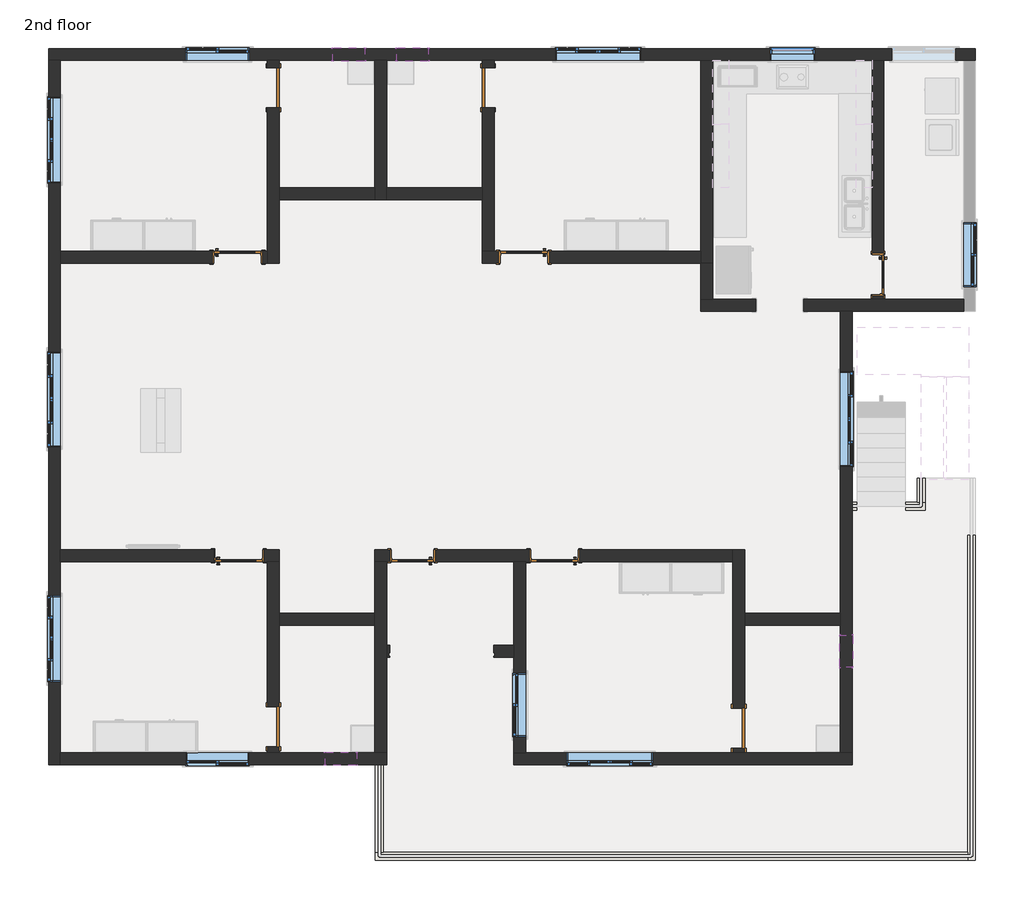
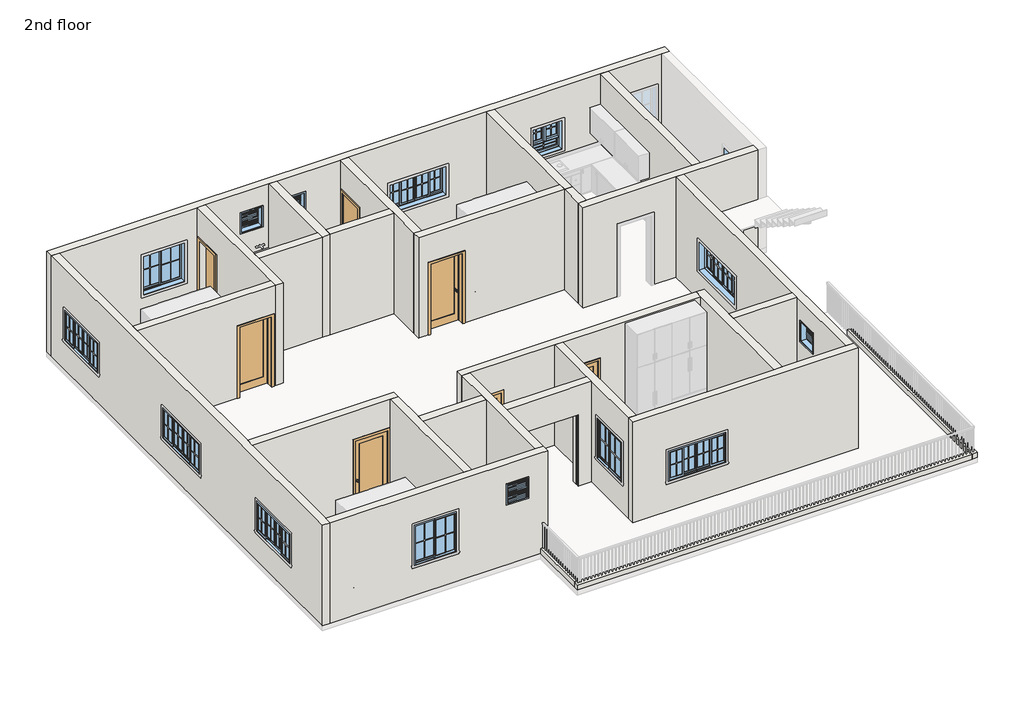
# One storey, part 1 of 4: 31 walls, 15 windows, 10 doors.
"""IFC4 building model written with IfcOpenShell, lengths in millimetres."""

from ifc_helpers import new_model, si_unit, frame, origin, place, context, project, spatial, polyline, outline, extrude, faceted_brep, transform, mapped, element, save
from components import door_ac3c0746, door_868ee8a9, door_3b97b8e7, door_c0815308, door_5e1232af, door_bb98abfd, window_ced37e8f, window_f2d8fef0, window_5af5dca6, window_95c4569f, window_58cce754

model = new_model("IFC4")

# Units and contexts
model_context = context("Model", 3, world=origin())
ifc_project = project(units=[si_unit("LENGTHUNIT", "METRE", prefix="MILLI")], contexts=[model_context])

# Site, building, storey
site = spatial("IfcSite", under=ifc_project)
building = spatial("IfcBuilding", under=site)
storey = spatial("IfcBuildingStorey", under=building, Name="2nd floor", Elevation=7010.4)

# Doors
placement = place(None, origin())
door_shape = door_ac3c0746(model_context)
element("IfcDoor", 1, ObjectType="Door-Interior-Single-1_Panel-Wood : 30\" x 84\"", at=placement, inside=storey, context=model_context, shape_type="MappedRepresentation", body=[
    mapped(door_shape, transform((7861.3010838, 2743.2660813, 7010.4), x_axis=(0.0, -1.0, 0.0), y_axis=(1.0, 0.0, 0.0), z_axis=(0.0, 0.0, 1.0))),
])
door_2_shape = door_868ee8a9(model_context)
element("IfcDoor", 2, ObjectType="Door-Interior-Single-1_Panel-Wood : 36\" x 84\"", at=placement, inside=storey, context=model_context, shape_type="MappedRepresentation", body=[
    mapped(door_2_shape, transform((1076.3260838, 3076.6410813, 7010.4), x_axis=(-1.0, 0.0, 0.0), y_axis=(0.0, -1.0, 0.0), z_axis=(0.0, 0.0, 1.0))),
])
element("IfcDoor", 3, ObjectType="Door-Interior-Single-1_Panel-Wood : 36\" x 84\"", at=placement, inside=storey, context=model_context, shape_type="MappedRepresentation", body=[
    mapped(door_2_shape, transform((-4384.6739162, -2644.7089187, 7010.4), x_axis=(1.0, 0.0, 0.0), y_axis=(0.0, 1.0, 0.0), z_axis=(0.0, 0.0, 1.0))),
])
door_3_shape = door_3b97b8e7(model_context)
element("IfcDoor", 4, ObjectType="Door-Interior-Single-1_Panel-Wood : 36\" x 84\"", at=placement, inside=storey, context=model_context, shape_type="MappedRepresentation", body=[
    mapped(door_3_shape, transform((1660.5260838, -2644.7089187, 7010.4), x_axis=(-1.0, 0.0, 0.0), y_axis=(0.0, -1.0, 0.0), z_axis=(0.0, 0.0, 1.0))),
])
element("IfcDoor", 5, ObjectType="Door-Interior-Single-1_Panel-Wood : 36\" x 84\"", at=placement, inside=storey, context=model_context, shape_type="MappedRepresentation", body=[
    mapped(door_3_shape, transform((-4410.0739162, 3076.6410813, 7010.4), x_axis=(1.0, 0.0, 0.0), y_axis=(0.0, 1.0, 0.0), z_axis=(0.0, 0.0, 1.0))),
])
door_4_shape = door_c0815308(model_context)
element("IfcDoor", 6, ObjectType="Door-Interior-Single-Full Glass-Wood : 32\" x 84\"", at=placement, inside=storey, context=model_context, shape_type="MappedRepresentation", body=[
    mapped(door_4_shape, transform((-1057.2739162, -2644.7089187, 7010.4), x_axis=(-1.0, 0.0, 0.0), y_axis=(0.0, -1.0, 0.0), z_axis=(0.0, 0.0, 1.0))),
])
door_5_shape = door_5e1232af(model_context)
element("IfcDoor", 7, ObjectType="Single-Flush : 30\" x 84\"", at=placement, inside=storey, context=model_context, shape_type="MappedRepresentation", body=[
    mapped(door_5_shape, transform((-3724.2739162, 6324.6660813, 7010.4), x_axis=(0.0, 1.0, 0.0), y_axis=(-1.0, 0.0, 0.0), z_axis=(0.0, 0.0, 1.0))),
])
door_6_shape = door_bb98abfd(model_context)
element("IfcDoor", 8, ObjectType="Single-Flush : 30\" x 84\"", at=placement, inside=storey, context=model_context, shape_type="MappedRepresentation", body=[
    mapped(door_6_shape, transform((390.5260838, 6324.6660813, 7010.4), x_axis=(0.0, 1.0, 0.0), y_axis=(-1.0, 0.0, 0.0), z_axis=(0.0, 0.0, 1.0))),
])
element("IfcDoor", 9, ObjectType="Single-Flush : 30\" x 84\"", at=placement, inside=storey, context=model_context, shape_type="MappedRepresentation", body=[
    mapped(door_6_shape, transform((-3724.2739162, -5918.1339187, 7010.4), x_axis=(0.0, -1.0, 0.0), y_axis=(1.0, 0.0, 0.0), z_axis=(0.0, 0.0, 1.0))),
])
element("IfcDoor", 10, ObjectType="Single-Flush : 30\" x 84\"", at=placement, inside=storey, context=model_context, shape_type="MappedRepresentation", body=[
    mapped(door_6_shape, transform((5191.1260838, -5943.5339187, 7010.4), x_axis=(0.0, -1.0, 0.0), y_axis=(1.0, 0.0, 0.0), z_axis=(0.0, 0.0, 1.0))),
])

# Walls
element("IfcWall", 11, ObjectType="Generic - 6\"", at=placement, inside=storey, context=model_context, shape_type="Brep", body=[
    faceted_brep([(9572.6260838, -8470.8339187, 7010.4), (9572.6260838, -8470.8339187, 7162.8), (9572.6260838, -8318.4339187, 7162.8), (9572.6260838, -2247.8339187, 7162.8), (9572.6260838, -2247.8339187, 7010.4), (9572.6260838, -8318.4339187, 7010.4), (9725.0260838, -8470.8339187, 7162.8), (9725.0260838, -8470.8339187, 7010.4), (9725.0260838, -2247.8339187, 7010.4), (9725.0260838, -2247.8339187, 7162.8)], [[[0, 1, 2, 3, 4, 5]], [[6, 7, 8, 9]], [[7, 0, 5, 4, 8]], [[1, 6, 9, 3, 2]], [[1, 0, 7, 6]], [[4, 3, 9, 8]]]),
])
element("IfcWall", 12, ObjectType="Generic - 6\"", at=placement, inside=storey, context=model_context, shape_type="Brep", body=[
    faceted_brep([(9572.6260838, -8318.4339187, 7010.4), (-1616.0739162, -8318.4339187, 7010.4), (-1768.4739162, -8318.4339187, 7010.4), (-1768.4739162, -8318.4339187, 7162.8), (-1616.0739162, -8318.4339187, 7162.8), (9572.6260838, -8318.4339187, 7162.8), (9572.6260838, -8470.8339187, 7010.4), (9572.6260838, -8470.8339187, 7162.8), (-1768.4739162, -8470.8339187, 7162.8), (-1768.4739162, -8470.8339187, 7010.4)], [[[0, 1, 2, 3, 4, 5]], [[6, 7, 8, 9]], [[2, 1, 0, 6, 9]], [[5, 4, 3, 8, 7]], [[0, 5, 7, 6]], [[3, 2, 9, 8]]]),
])
element("IfcWall", 13, ObjectType="Generic - 6\"", at=placement, inside=storey, context=model_context, shape_type="SweptSolid", body=[
    extrude(outline(polyline([(-1616.0739162, -6642.0339187), (-1616.0739162, -8318.4339187), (-1768.4739162, -8318.4339187), (-1768.4739162, -6642.0339187), (-1616.0739162, -6642.0339187)])), frame((0.0, 0.0, 7010.4), z_axis=(0.0, 0.0, 1.0), x_axis=(1.0, 0.0, 0.0)), (0.0, 0.0, 1.0), 152.4),
])
element("IfcWall", 14, ObjectType="Generic - 6\"", at=placement, inside=storey, context=model_context, shape_type="SweptSolid", body=[
    extrude(outline(polyline([(8607.4260838, -1612.8339187), (8607.4260838, -1156.9972984), (8759.8260838, -1156.9972984), (8759.8260838, -1612.8339187), (8607.4260838, -1612.8339187)])), frame((0.0, 0.0, 7010.4), z_axis=(0.0, 0.0, 1.0), x_axis=(1.0, 0.0, 0.0)), (0.0, 0.0, 1.0), 152.4),
])
element("IfcWall", 15, ObjectType="Generic - 6\"", at=placement, inside=storey, context=model_context, shape_type="Brep", body=[
    faceted_brep([(8759.8260838, -1612.8339187, 7010.4), (8607.4260838, -1612.8339187, 7010.4), (8391.5260838, -1612.8339187, 7010.4), (8391.5260838, -1612.8339187, 7162.8), (8607.4260838, -1612.8339187, 7162.8), (8759.8260838, -1612.8339187, 7162.8), (8759.8260838, -1765.2339187, 7010.4), (8759.8260838, -1765.2339187, 7162.8), (8391.5260838, -1765.2339187, 7162.8), (8391.5260838, -1765.2339187, 7010.4)], [[[0, 1, 2, 3, 4, 5]], [[6, 7, 8, 9]], [[2, 1, 0, 6, 9]], [[3, 2, 9, 8]], [[5, 4, 3, 8, 7]], [[0, 5, 7, 6]]]),
])
element("IfcWall", 16, ObjectType="Generic - 6\"", at=placement, inside=storey, context=model_context, shape_type="SweptSolid", body=[
    extrude(outline(polyline([(7362.8260838, -1612.8339187), (7451.7260838, -1612.8339187), (7451.7260838, -1765.2339187), (7362.8260838, -1765.2339187), (7362.8260838, -1612.8339187)])), frame((0.0, 0.0, 7010.4), z_axis=(0.0, 0.0, 1.0), x_axis=(1.0, 0.0, 0.0)), (0.0, 0.0, 1.0), 152.4),
])
element("IfcWall", 17, ObjectType="Generic - 9\"", at=placement, inside=storey, context=model_context, shape_type="Brep", body=[
    faceted_brep([(-8029.5739162, 6845.3660813, 7010.4), (-7800.9739162, 6845.3660813, 7010.4), (-3838.5739162, 6845.3660813, 7010.4), (-3609.9739162, 6845.3660813, 7010.4), (-1781.1739162, 6845.3660813, 7010.4), (-1552.5739162, 6845.3660813, 7010.4), (276.2260838, 6845.3660813, 7010.4), (504.8260838, 6845.3660813, 7010.4), (4467.2260838, 6845.3660813, 7010.4), (4695.8260838, 6845.3660813, 7010.4), (7743.8260838, 6845.3660813, 7010.4), (7972.4260838, 6845.3660813, 7010.4), (9496.4260838, 6845.3660813, 7010.4), (9725.0260838, 6845.3660813, 7010.4), (9725.0260838, 6845.3660813, 10058.4), (9496.4260838, 6845.3660813, 10058.4), (7972.4260838, 6845.3660813, 10058.4), (7743.8260838, 6845.3660813, 10058.4), (4695.8260838, 6845.3660813, 10058.4), (4467.2260838, 6845.3660813, 10058.4), (504.8260838, 6845.3660813, 10058.4), (276.2260838, 6845.3660813, 10058.4), (-1552.5739162, 6845.3660813, 10058.4), (-1781.1739162, 6845.3660813, 10058.4), (-3609.9739162, 6845.3660813, 10058.4), (-3838.5739162, 6845.3660813, 10058.4), (-7800.9739162, 6845.3660813, 10058.4), (-8029.5739162, 6845.3660813, 10058.4), (3324.2260838, 6845.3660813, 8839.2), (3324.2260838, 6845.3660813, 7924.8), (1673.2260838, 6845.3660813, 7924.8), (1673.2260838, 6845.3660813, 8839.2), (9344.0260838, 6845.3660813, 9144.0), (9344.0260838, 6845.3660813, 7924.8), (8124.8260838, 6845.3660813, 7924.8), (8124.8260838, 6845.3660813, 9144.0), (-2581.2739162, 6845.3660813, 9448.8), (-1971.6739162, 6845.3660813, 9448.8), (-1971.6739162, 6845.3660813, 8839.2), (-2581.2739162, 6845.3660813, 8839.2), (-1362.0739162, 6845.3660813, 9448.8), (-752.4739162, 6845.3660813, 9448.8), (-752.4739162, 6845.3660813, 8839.2), (-1362.0739162, 6845.3660813, 8839.2), (-4181.4739162, 6845.3660813, 9144.0), (-4181.4739162, 6845.3660813, 7924.8), (-5400.6739162, 6845.3660813, 7924.8), (-5400.6739162, 6845.3660813, 9144.0), (6651.6260838, 6845.3660813, 9067.8), (6651.6260838, 6845.3660813, 8153.4), (5788.0260838, 6845.3660813, 8153.4), (5788.0260838, 6845.3660813, 9067.8), (-8029.5739162, 7073.9660813, 7010.4), (-8029.5739162, 7073.9660813, 10058.4), (9725.0260838, 7073.9660813, 10058.4), (9725.0260838, 7073.9660813, 7010.4), (3324.2260838, 7073.9660813, 8839.2), (1673.2260838, 7073.9660813, 8839.2), (1673.2260838, 7073.9660813, 7924.8), (3324.2260838, 7073.9660813, 7924.8), (9344.0260838, 7073.9660813, 9144.0), (8124.8260838, 7073.9660813, 9144.0), (8124.8260838, 7073.9660813, 7924.8), (9344.0260838, 7073.9660813, 7924.8), (-2581.2739162, 7073.9660813, 9448.8), (-2581.2739162, 7073.9660813, 8839.2), (-1971.6739162, 7073.9660813, 8839.2), (-1971.6739162, 7073.9660813, 9448.8), (-1362.0739162, 7073.9660813, 9448.8), (-1362.0739162, 7073.9660813, 8839.2), (-752.4739162, 7073.9660813, 8839.2), (-752.4739162, 7073.9660813, 9448.8), (-4181.4739162, 7073.9660813, 9144.0), (-5400.6739162, 7073.9660813, 9144.0), (-5400.6739162, 7073.9660813, 7924.8), (-4181.4739162, 7073.9660813, 7924.8), (6651.6260838, 7073.9660813, 9067.8), (5788.0260838, 7073.9660813, 9067.8), (5788.0260838, 7073.9660813, 8153.4), (6651.6260838, 7073.9660813, 8153.4)], [[[0, 1, 2, 3, 4, 5, 6, 7, 8, 9, 10, 11, 12, 13, 14, 15, 16, 17, 18, 19, 20, 21, 22, 23, 24, 25, 26, 27], [28, 29, 30, 31], [32, 33, 34, 35], [36, 37, 38, 39], [40, 41, 42, 43], [44, 45, 46, 47], [48, 49, 50, 51]], [[52, 53, 54, 55], [56, 57, 58, 59], [60, 61, 62, 63], [64, 65, 66, 67], [68, 69, 70, 71], [72, 73, 74, 75], [76, 77, 78, 79]], [[13, 12, 11, 10, 9, 8, 7, 6, 5, 4, 3, 2, 1, 0, 52, 55]], [[0, 27, 53, 52]], [[14, 13, 55, 54]], [[29, 28, 56, 59]], [[30, 29, 59, 58]], [[31, 30, 58, 57]], [[28, 31, 57, 56]], [[33, 32, 60, 63]], [[34, 33, 63, 62]], [[35, 34, 62, 61]], [[32, 35, 61, 60]], [[65, 64, 36, 39]], [[66, 65, 39, 38]], [[67, 66, 38, 37]], [[64, 67, 37, 36]], [[69, 68, 40, 43]], [[70, 69, 43, 42]], [[71, 70, 42, 41]], [[68, 71, 41, 40]], [[45, 44, 72, 75]], [[46, 45, 75, 74]], [[47, 46, 74, 73]], [[44, 47, 73, 72]], [[49, 48, 76, 79]], [[50, 49, 79, 78]], [[51, 50, 78, 77]], [[48, 51, 77, 76]], [[27, 26, 25, 24, 23, 22, 21, 20, 19, 18, 17, 16, 15, 14, 54, 53]]]),
])
element("IfcWall", 18, ObjectType="Generic - 9\"", at=placement, inside=storey, context=model_context, shape_type="Brep", body=[
    faceted_brep([(-8029.5739162, 6845.3660813, 7010.4), (-8029.5739162, -6642.0339187, 7010.4), (-8029.5739162, -6642.0339187, 10058.4), (-8029.5739162, 6845.3660813, 10058.4), (-8029.5739162, 1270.0660813, 8839.2), (-8029.5739162, -558.7339187, 8839.2), (-8029.5739162, -558.7339187, 7924.8), (-8029.5739162, 1270.0660813, 7924.8), (-8029.5739162, 6146.8660813, 8839.2), (-8029.5739162, 4495.8660813, 8839.2), (-8029.5739162, 4495.8660813, 7924.8), (-8029.5739162, 6146.8660813, 7924.8), (-8029.5739162, -3403.5339187, 8839.2), (-8029.5739162, -5054.5339187, 8839.2), (-8029.5739162, -5054.5339187, 7924.8), (-8029.5739162, -3403.5339187, 7924.8), (-7800.9739162, 6845.3660813, 7010.4), (-7800.9739162, 6845.3660813, 10058.4), (-7800.9739162, 3187.7660813, 10058.4), (-7800.9739162, 2959.1660813, 10058.4), (-7800.9739162, -2527.2339187, 10058.4), (-7800.9739162, -2755.8339187, 10058.4), (-7800.9739162, -6413.4339187, 10058.4), (-7800.9739162, -6642.0339187, 10058.4), (-7800.9739162, -6642.0339187, 7010.4), (-7800.9739162, -6413.4339187, 7010.4), (-7800.9739162, -2755.8339187, 7010.4), (-7800.9739162, -2527.2339187, 7010.4), (-7800.9739162, 2959.1660813, 7010.4), (-7800.9739162, 3187.7660813, 7010.4), (-7800.9739162, 1270.0660813, 8839.2), (-7800.9739162, 1270.0660813, 7924.8), (-7800.9739162, -558.7339187, 7924.8), (-7800.9739162, -558.7339187, 8839.2), (-7800.9739162, 6146.8660813, 8839.2), (-7800.9739162, 6146.8660813, 7924.8), (-7800.9739162, 4495.8660813, 7924.8), (-7800.9739162, 4495.8660813, 8839.2), (-7800.9739162, -3403.5339187, 8839.2), (-7800.9739162, -3403.5339187, 7924.8), (-7800.9739162, -5054.5339187, 7924.8), (-7800.9739162, -5054.5339187, 8839.2)], [[[0, 1, 2, 3], [4, 5, 6, 7], [8, 9, 10, 11], [12, 13, 14, 15]], [[16, 17, 18, 19, 20, 21, 22, 23, 24, 25, 26, 27, 28, 29], [30, 31, 32, 33], [34, 35, 36, 37], [38, 39, 40, 41]], [[1, 0, 16, 29, 28, 27, 26, 25, 24]], [[0, 3, 17, 16]], [[2, 1, 24, 23]], [[31, 30, 4, 7]], [[32, 31, 7, 6]], [[33, 32, 6, 5]], [[30, 33, 5, 4]], [[35, 34, 8, 11]], [[36, 35, 11, 10]], [[37, 36, 10, 9]], [[34, 37, 9, 8]], [[39, 38, 12, 15]], [[40, 39, 15, 14]], [[41, 40, 14, 13]], [[38, 41, 13, 12]], [[3, 2, 23, 22, 21, 20, 19, 18, 17]]]),
])
element("IfcWall", 19, ObjectType="Generic - 9\"", at=placement, inside=storey, context=model_context, shape_type="Brep", body=[
    faceted_brep([(-3838.5739162, 6845.3660813, 10058.4), (-3838.5739162, 6845.3660813, 7010.4), (-3838.5739162, 6705.6660813, 7010.4), (-3838.5739162, 6705.6660813, 9144.0), (-3838.5739162, 5943.6660813, 9144.0), (-3838.5739162, 5943.6660813, 7010.4), (-3838.5739162, 3187.7660813, 7010.4), (-3838.5739162, 2959.1660813, 7010.4), (-3838.5739162, 2959.1660813, 10058.4), (-3838.5739162, 3187.7660813, 10058.4), (-3609.9739162, 6845.3660813, 7010.4), (-3609.9739162, 6845.3660813, 10058.4), (-3609.9739162, 4406.9660813, 10058.4), (-3609.9739162, 4178.3660813, 10058.4), (-3609.9739162, 2959.1660813, 10058.4), (-3609.9739162, 2959.1660813, 7010.4), (-3609.9739162, 4178.3660813, 7010.4), (-3609.9739162, 4406.9660813, 7010.4), (-3609.9739162, 5943.6660813, 7010.4), (-3609.9739162, 5943.6660813, 9144.0), (-3609.9739162, 6705.6660813, 9144.0), (-3609.9739162, 6705.6660813, 7010.4)], [[[0, 1, 2, 3, 4, 5, 6, 7, 8, 9]], [[10, 11, 12, 13, 14, 15, 16, 17, 18, 19, 20, 21]], [[1, 10, 21, 2]], [[15, 7, 6, 5, 18, 17, 16]], [[1, 0, 11, 10]], [[8, 7, 15, 14]], [[20, 3, 2, 21]], [[4, 19, 18, 5]], [[19, 4, 3, 20]], [[0, 9, 8, 14, 13, 12, 11]]]),
])
element("IfcWall", 20, ObjectType="Generic - 9\"", at=placement, inside=storey, context=model_context, shape_type="Brep", body=[
    faceted_brep([(-1781.1739162, 6845.3660813, 7010.4), (-1781.1739162, 4406.9660813, 7010.4), (-1781.1739162, 4178.3660813, 7010.4), (-1781.1739162, 4178.3660813, 10058.4), (-1781.1739162, 4406.9660813, 10058.4), (-1781.1739162, 6845.3660813, 10058.4), (-1552.5739162, 6845.3660813, 7010.4), (-1552.5739162, 6845.3660813, 10058.4), (-1552.5739162, 4406.9660813, 10058.4), (-1552.5739162, 4178.3660813, 10058.4), (-1552.5739162, 4178.3660813, 7010.4), (-1552.5739162, 4406.9660813, 7010.4)], [[[0, 1, 2, 3, 4, 5]], [[6, 7, 8, 9, 10, 11]], [[2, 1, 0, 6, 11, 10]], [[0, 5, 7, 6]], [[3, 2, 10, 9]], [[5, 4, 3, 9, 8, 7]]]),
])
element("IfcWall", 21, ObjectType="Generic - 9\"", at=placement, inside=storey, context=model_context, shape_type="Brep", body=[
    faceted_brep([(276.2260838, 6845.3660813, 10058.4), (276.2260838, 6845.3660813, 7010.4), (276.2260838, 6705.6660813, 7010.4), (276.2260838, 6705.6660813, 9144.0), (276.2260838, 5943.6660813, 9144.0), (276.2260838, 5943.6660813, 7010.4), (276.2260838, 4406.9660813, 7010.4), (276.2260838, 4178.3660813, 7010.4), (276.2260838, 3187.7660813, 7010.4), (276.2260838, 3187.7660813, 10058.4), (276.2260838, 4178.3660813, 10058.4), (276.2260838, 4406.9660813, 10058.4), (504.8260838, 6845.3660813, 7010.4), (504.8260838, 6845.3660813, 10058.4), (504.8260838, 3187.7660813, 10058.4), (504.8260838, 3187.7660813, 7010.4), (504.8260838, 5943.6660813, 7010.4), (504.8260838, 5943.6660813, 9144.0), (504.8260838, 6705.6660813, 9144.0), (504.8260838, 6705.6660813, 7010.4)], [[[0, 1, 2, 3, 4, 5, 6, 7, 8, 9, 10, 11]], [[12, 13, 14, 15, 16, 17, 18, 19]], [[1, 12, 19, 2]], [[15, 8, 7, 6, 5, 16]], [[1, 0, 13, 12]], [[9, 8, 15, 14]], [[18, 3, 2, 19]], [[4, 17, 16, 5]], [[17, 4, 3, 18]], [[0, 11, 10, 9, 14, 13]]]),
])
element("IfcWall", 22, ObjectType="Generic - 9\"", at=placement, inside=storey, context=model_context, shape_type="Brep", body=[
    faceted_brep([(4467.2260838, 6845.3660813, 7010.4), (4467.2260838, 3187.7660813, 7010.4), (4467.2260838, 2959.1660813, 7010.4), (4467.2260838, 2959.1660813, 10058.4), (4467.2260838, 3187.7660813, 10058.4), (4467.2260838, 6845.3660813, 10058.4), (4695.8260838, 6845.3660813, 7010.4), (4695.8260838, 6845.3660813, 10058.4), (4695.8260838, 2959.1660813, 10058.4), (4695.8260838, 2959.1660813, 7010.4)], [[[0, 1, 2, 3, 4, 5]], [[6, 7, 8, 9]], [[2, 1, 0, 6, 9]], [[3, 2, 9, 8]], [[0, 5, 7, 6]], [[5, 4, 3, 8, 7]]]),
])
element("IfcWall", 23, ObjectType="Generic - 9\"", at=placement, inside=storey, context=model_context, shape_type="SweptSolid", body=[
    extrude(outline(polyline([(7010.4, -3838.5739162), (10058.4, -3838.5739162), (10058.4, -7800.9739162), (7010.4, -7800.9739162), (7010.4, -4892.6739162), (9169.4, -4892.6739162), (9169.4, -3927.4739162), (7010.4, -3927.4739162), (7010.4, -3838.5739162)])), frame((0.0, 2959.1660813, 0.0), z_axis=(0.0, 1.0, 0.0), x_axis=(0.0, 0.0, 1.0)), (0.0, 0.0, 1.0), 228.6),
])
element("IfcWall", 24, ObjectType="Generic - 9\"", at=placement, inside=storey, context=model_context, shape_type="SweptSolid", body=[
    extrude(outline(polyline([(-3609.9739162, 4406.9660813), (-1781.1739162, 4406.9660813), (-1781.1739162, 4178.3660813), (-3609.9739162, 4178.3660813), (-3609.9739162, 4406.9660813)])), frame((0.0, 0.0, 7010.4), z_axis=(0.0, 0.0, 1.0), x_axis=(1.0, 0.0, 0.0)), (0.0, 0.0, 1.0), 3048.0),
])
element("IfcWall", 25, ObjectType="Generic - 9\"", at=placement, inside=storey, context=model_context, shape_type="SweptSolid", body=[
    extrude(outline(polyline([(276.2260838, 4178.3660813), (-1552.5739162, 4178.3660813), (-1552.5739162, 4406.9660813), (276.2260838, 4406.9660813), (276.2260838, 4178.3660813)])), frame((0.0, 0.0, 7010.4), z_axis=(0.0, 0.0, 1.0), x_axis=(1.0, 0.0, 0.0)), (0.0, 0.0, 1.0), 3048.0),
])
element("IfcWall", 26, ObjectType="Generic - 9\"", at=placement, inside=storey, context=model_context, shape_type="Brep", body=[
    faceted_brep([(4467.2260838, 2959.1660813, 7010.4), (4467.2260838, 2959.1660813, 10058.4), (276.2260838, 2959.1660813, 10058.4), (276.2260838, 2959.1660813, 7010.4), (593.7260838, 2959.1660813, 7010.4), (593.7260838, 2959.1660813, 9169.4), (1558.9260838, 2959.1660813, 9169.4), (1558.9260838, 2959.1660813, 7010.4), (4467.2260838, 3187.7660813, 10058.4), (4467.2260838, 3187.7660813, 7010.4), (1558.9260838, 3187.7660813, 7010.4), (1558.9260838, 3187.7660813, 9169.4), (593.7260838, 3187.7660813, 9169.4), (593.7260838, 3187.7660813, 7010.4), (504.8260838, 3187.7660813, 7010.4), (276.2260838, 3187.7660813, 7010.4), (276.2260838, 3187.7660813, 10058.4), (504.8260838, 3187.7660813, 10058.4)], [[[0, 1, 2, 3, 4, 5, 6, 7]], [[8, 9, 10, 11, 12, 13, 14, 15, 16, 17]], [[9, 0, 7, 10]], [[3, 15, 14, 13, 4]], [[1, 0, 9, 8]], [[3, 2, 16, 15]], [[12, 5, 4, 13]], [[5, 12, 11, 6]], [[6, 11, 10, 7]], [[2, 1, 8, 17, 16]]]),
])
element("IfcWall", 27, ObjectType="Generic - 9\"", at=placement, inside=storey, context=model_context, shape_type="Brep", body=[
    faceted_brep([(-7800.9739162, -2755.8339187, 10058.4), (-7800.9739162, -2755.8339187, 7010.4), (-4867.2739162, -2755.8339187, 7010.4), (-4867.2739162, -2755.8339187, 9169.4), (-3902.0739162, -2755.8339187, 9169.4), (-3902.0739162, -2755.8339187, 7010.4), (-3838.5739162, -2755.8339187, 7010.4), (-3609.9739162, -2755.8339187, 7010.4), (-3609.9739162, -2755.8339187, 10058.4), (-3838.5739162, -2755.8339187, 10058.4), (-7800.9739162, -2527.2339187, 7010.4), (-7800.9739162, -2527.2339187, 10058.4), (-3609.9739162, -2527.2339187, 10058.4), (-3609.9739162, -2527.2339187, 7010.4), (-3902.0739162, -2527.2339187, 7010.4), (-3902.0739162, -2527.2339187, 9169.4), (-4867.2739162, -2527.2339187, 9169.4), (-4867.2739162, -2527.2339187, 7010.4)], [[[0, 1, 2, 3, 4, 5, 6, 7, 8, 9]], [[10, 11, 12, 13, 14, 15, 16, 17]], [[1, 10, 17, 2]], [[13, 7, 6, 5, 14]], [[1, 0, 11, 10]], [[8, 7, 13, 12]], [[4, 15, 14, 5]], [[15, 4, 3, 16]], [[16, 3, 2, 17]], [[0, 9, 8, 12, 11]]]),
])
element("IfcWall", 28, ObjectType="Generic - 9\"", at=placement, inside=storey, context=model_context, shape_type="Brep", body=[
    faceted_brep([(-7800.9739162, -6642.0339187, 7010.4), (-1768.4739162, -6642.0339187, 7010.4), (-1616.0739162, -6642.0339187, 7010.4), (-1552.5739162, -6642.0339187, 7010.4), (-1552.5739162, -6642.0339187, 10058.4), (-1781.1739162, -6642.0339187, 10058.4), (-7800.9739162, -6642.0339187, 10058.4), (-5400.6739162, -6642.0339187, 7924.8), (-5400.6739162, -6642.0339187, 9144.0), (-4181.4739162, -6642.0339187, 9144.0), (-4181.4739162, -6642.0339187, 7924.8), (-2124.0739162, -6642.0339187, 9448.8), (-2124.0739162, -6642.0339187, 8839.2), (-2733.6739162, -6642.0339187, 8839.2), (-2733.6739162, -6642.0339187, 9448.8), (-1552.5739162, -6413.4339187, 7010.4), (-1781.1739162, -6413.4339187, 7010.4), (-3609.9739162, -6413.4339187, 7010.4), (-3838.5739162, -6413.4339187, 7010.4), (-7800.9739162, -6413.4339187, 7010.4), (-7800.9739162, -6413.4339187, 10058.4), (-3838.5739162, -6413.4339187, 10058.4), (-3609.9739162, -6413.4339187, 10058.4), (-1781.1739162, -6413.4339187, 10058.4), (-1552.5739162, -6413.4339187, 10058.4), (-5400.6739162, -6413.4339187, 9144.0), (-5400.6739162, -6413.4339187, 7924.8), (-4181.4739162, -6413.4339187, 7924.8), (-4181.4739162, -6413.4339187, 9144.0), (-2124.0739162, -6413.4339187, 8839.2), (-2124.0739162, -6413.4339187, 9448.8), (-2733.6739162, -6413.4339187, 9448.8), (-2733.6739162, -6413.4339187, 8839.2)], [[[0, 1, 2, 3, 4, 5, 6], [7, 8, 9, 10], [11, 12, 13, 14]], [[15, 16, 17, 18, 19, 20, 21, 22, 23, 24], [25, 26, 27, 28], [29, 30, 31, 32]], [[3, 2, 1, 0, 19, 18, 17, 16, 15]], [[0, 6, 20, 19]], [[25, 8, 7, 26]], [[26, 7, 10, 27]], [[27, 10, 9, 28]], [[8, 25, 28, 9]], [[12, 11, 30, 29]], [[13, 12, 29, 32]], [[14, 13, 32, 31]], [[11, 14, 31, 30]], [[3, 15, 24, 4]], [[24, 23, 22, 21, 20, 6, 5, 4]]]),
])
element("IfcWall", 29, ObjectType="Generic - 9\"", at=placement, inside=storey, context=model_context, shape_type="Brep", body=[
    faceted_brep([(-3609.9739162, -6413.4339187, 10058.4), (-3609.9739162, -6413.4339187, 7010.4), (-3609.9739162, -6299.1339187, 7010.4), (-3609.9739162, -6299.1339187, 9144.0), (-3609.9739162, -5537.1339187, 9144.0), (-3609.9739162, -5537.1339187, 7010.4), (-3609.9739162, -3975.0339187, 7010.4), (-3609.9739162, -3746.4339187, 7010.4), (-3609.9739162, -2755.8339187, 7010.4), (-3609.9739162, -2755.8339187, 10058.4), (-3609.9739162, -3746.4339187, 10058.4), (-3609.9739162, -3975.0339187, 10058.4), (-3838.5739162, -6413.4339187, 7010.4), (-3838.5739162, -6413.4339187, 10058.4), (-3838.5739162, -2755.8339187, 10058.4), (-3838.5739162, -2755.8339187, 7010.4), (-3838.5739162, -5537.1339187, 7010.4), (-3838.5739162, -5537.1339187, 9144.0), (-3838.5739162, -6299.1339187, 9144.0), (-3838.5739162, -6299.1339187, 7010.4)], [[[0, 1, 2, 3, 4, 5, 6, 7, 8, 9, 10, 11]], [[12, 13, 14, 15, 16, 17, 18, 19]], [[1, 12, 19, 2]], [[15, 8, 7, 6, 5, 16]], [[1, 0, 13, 12]], [[9, 8, 15, 14]], [[18, 3, 2, 19]], [[4, 17, 16, 5]], [[17, 4, 3, 18]], [[0, 11, 10, 9, 14, 13]]]),
])
element("IfcWall", 30, ObjectType="Generic - 9\"", at=placement, inside=storey, context=model_context, shape_type="Brep", body=[
    faceted_brep([(-1781.1739162, -2755.8339187, 7010.4), (-1781.1739162, -3746.4339187, 7010.4), (-1781.1739162, -3975.0339187, 7010.4), (-1781.1739162, -6413.4339187, 7010.4), (-1781.1739162, -6413.4339187, 10058.4), (-1781.1739162, -3975.0339187, 10058.4), (-1781.1739162, -3746.4339187, 10058.4), (-1781.1739162, -2755.8339187, 10058.4), (-1552.5739162, -2755.8339187, 7010.4), (-1552.5739162, -2755.8339187, 10058.4), (-1552.5739162, -4356.0339187, 10058.4), (-1552.5739162, -4584.6339187, 10058.4), (-1552.5739162, -6413.4339187, 10058.4), (-1552.5739162, -6413.4339187, 7010.4), (-1552.5739162, -4584.6339187, 7010.4), (-1552.5739162, -4356.0339187, 7010.4)], [[[0, 1, 2, 3, 4, 5, 6, 7]], [[8, 9, 10, 11, 12, 13, 14, 15]], [[3, 2, 1, 0, 8, 15, 14, 13]], [[0, 7, 9, 8]], [[7, 6, 5, 4, 12, 11, 10, 9]], [[3, 13, 12, 4]]]),
])
element("IfcWall", 31, ObjectType="Generic - 9\"", at=placement, inside=storey, context=model_context, shape_type="SweptSolid", body=[
    extrude(outline(polyline([(-3609.9739162, -3746.4339187), (-1781.1739162, -3746.4339187), (-1781.1739162, -3975.0339187), (-3609.9739162, -3975.0339187), (-3609.9739162, -3746.4339187)])), frame((0.0, 0.0, 7010.4), z_axis=(0.0, 0.0, 1.0), x_axis=(1.0, 0.0, 0.0)), (0.0, 0.0, 1.0), 3048.0),
])
element("IfcWall", 32, ObjectType="Generic - 9\"", at=placement, inside=storey, context=model_context, shape_type="Brep", body=[
    faceted_brep([(1114.4260838, -6413.4339187, 7010.4), (1114.4260838, -2755.8339187, 7010.4), (1114.4260838, -2755.8339187, 10058.4), (1114.4260838, -6413.4339187, 10058.4), (1114.4260838, -4889.4339187, 9144.0), (1114.4260838, -4889.4339187, 7924.8), (1114.4260838, -6108.6339187, 7924.8), (1114.4260838, -6108.6339187, 9144.0), (885.8260838, -2755.8339187, 7010.4), (885.8260838, -4356.0339187, 7010.4), (885.8260838, -4584.6339187, 7010.4), (885.8260838, -6413.4339187, 7010.4), (885.8260838, -6413.4339187, 10058.4), (885.8260838, -4584.6339187, 10058.4), (885.8260838, -4356.0339187, 10058.4), (885.8260838, -2755.8339187, 10058.4), (885.8260838, -4889.4339187, 7924.8), (885.8260838, -4889.4339187, 9144.0), (885.8260838, -6108.6339187, 9144.0), (885.8260838, -6108.6339187, 7924.8)], [[[0, 1, 2, 3], [4, 5, 6, 7]], [[8, 9, 10, 11, 12, 13, 14, 15], [16, 17, 18, 19]], [[1, 0, 11, 10, 9, 8]], [[2, 1, 8, 15]], [[0, 3, 12, 11]], [[4, 17, 16, 5]], [[5, 16, 19, 6]], [[6, 19, 18, 7]], [[17, 4, 7, 18]], [[3, 2, 15, 14, 13, 12]]]),
])
element("IfcWall", 33, ObjectType="Generic - 9\"", at=placement, inside=storey, context=model_context, shape_type="Brep", body=[
    faceted_brep([(-1781.1739162, -2527.2339187, 7010.4), (-1781.1739162, -2527.2339187, 10058.4), (5076.8260838, -2527.2339187, 10058.4), (5076.8260838, -2527.2339187, 7010.4), (2143.1260838, -2527.2339187, 7010.4), (2143.1260838, -2527.2339187, 9169.4), (1177.9260838, -2527.2339187, 9169.4), (1177.9260838, -2527.2339187, 7010.4), (-625.4739162, -2527.2339187, 7010.4), (-625.4739162, -2527.2339187, 9169.4), (-1489.0739162, -2527.2339187, 9169.4), (-1489.0739162, -2527.2339187, 7010.4), (-1781.1739162, -2755.8339187, 10058.4), (-1781.1739162, -2755.8339187, 7010.4), (-1552.5739162, -2755.8339187, 7010.4), (-1489.0739162, -2755.8339187, 7010.4), (-1489.0739162, -2755.8339187, 9169.4), (-625.4739162, -2755.8339187, 9169.4), (-625.4739162, -2755.8339187, 7010.4), (885.8260838, -2755.8339187, 7010.4), (1114.4260838, -2755.8339187, 7010.4), (1177.9260838, -2755.8339187, 7010.4), (1177.9260838, -2755.8339187, 9169.4), (2143.1260838, -2755.8339187, 9169.4), (2143.1260838, -2755.8339187, 7010.4), (5076.8260838, -2755.8339187, 7010.4), (5076.8260838, -2755.8339187, 10058.4), (1114.4260838, -2755.8339187, 10058.4), (885.8260838, -2755.8339187, 10058.4), (-1552.5739162, -2755.8339187, 10058.4)], [[[0, 1, 2, 3, 4, 5, 6, 7, 8, 9, 10, 11]], [[12, 13, 14, 15, 16, 17, 18, 19, 20, 21, 22, 23, 24, 25, 26, 27, 28, 29]], [[13, 0, 11, 15, 14]], [[3, 25, 24, 4]], [[7, 21, 20, 19, 18, 8]], [[1, 0, 13, 12]], [[3, 2, 26, 25]], [[6, 22, 21, 7]], [[22, 6, 5, 23]], [[23, 5, 4, 24]], [[10, 16, 15, 11]], [[16, 10, 9, 17]], [[17, 9, 8, 18]], [[2, 1, 12, 29, 28, 27, 26]]]),
])
element("IfcWall", 34, ObjectType="Generic - 9\"", at=placement, inside=storey, context=model_context, shape_type="Brep", body=[
    faceted_brep([(5305.4260838, -6413.4339187, 10058.4), (5305.4260838, -6413.4339187, 7010.4), (5305.4260838, -6324.5339187, 7010.4), (5305.4260838, -6324.5339187, 9144.0), (5305.4260838, -5562.5339187, 9144.0), (5305.4260838, -5562.5339187, 7010.4), (5305.4260838, -3975.0339187, 7010.4), (5305.4260838, -3746.4339187, 7010.4), (5305.4260838, -2527.2339187, 7010.4), (5305.4260838, -2527.2339187, 10058.4), (5305.4260838, -3746.4339187, 10058.4), (5305.4260838, -3975.0339187, 10058.4), (5076.8260838, -6413.4339187, 7010.4), (5076.8260838, -6413.4339187, 10058.4), (5076.8260838, -2755.8339187, 10058.4), (5076.8260838, -2527.2339187, 10058.4), (5076.8260838, -2527.2339187, 7010.4), (5076.8260838, -2755.8339187, 7010.4), (5076.8260838, -5562.5339187, 7010.4), (5076.8260838, -5562.5339187, 9144.0), (5076.8260838, -6324.5339187, 9144.0), (5076.8260838, -6324.5339187, 7010.4)], [[[0, 1, 2, 3, 4, 5, 6, 7, 8, 9, 10, 11]], [[12, 13, 14, 15, 16, 17, 18, 19, 20, 21]], [[1, 12, 21, 2]], [[16, 8, 7, 6, 5, 18, 17]], [[1, 0, 13, 12]], [[9, 8, 16, 15]], [[20, 3, 2, 21]], [[4, 19, 18, 5]], [[19, 4, 3, 20]], [[0, 11, 10, 9, 15, 14, 13]]]),
])
element("IfcWall", 35, ObjectType="Generic - 9\"", at=placement, inside=storey, context=model_context, shape_type="Brep", body=[
    faceted_brep([(7362.8260838, -6413.4339187, 7010.4), (7362.8260838, -1765.2339187, 7010.4), (7362.8260838, -1612.8339187, 7010.4), (7362.8260838, 2044.7660813, 7010.4), (7362.8260838, 2044.7660813, 10058.4), (7362.8260838, -1689.0339187, 10058.4), (7362.8260838, -6413.4339187, 10058.4), (7362.8260838, -939.7339187, 7924.8), (7362.8260838, -939.7339187, 8839.2), (7362.8260838, 889.0660813, 8839.2), (7362.8260838, 889.0660813, 7924.8), (7362.8260838, -4165.5339187, 9448.8), (7362.8260838, -4165.5339187, 8839.2), (7362.8260838, -4775.1339187, 8839.2), (7362.8260838, -4775.1339187, 9448.8), (7134.2260838, 2044.7660813, 7010.4), (7134.2260838, -3746.4339187, 7010.4), (7134.2260838, -3975.0339187, 7010.4), (7134.2260838, -6413.4339187, 7010.4), (7134.2260838, -6413.4339187, 10058.4), (7134.2260838, -3975.0339187, 10058.4), (7134.2260838, -3746.4339187, 10058.4), (7134.2260838, 2044.7660813, 10058.4), (7134.2260838, -939.7339187, 8839.2), (7134.2260838, -939.7339187, 7924.8), (7134.2260838, 889.0660813, 7924.8), (7134.2260838, 889.0660813, 8839.2), (7134.2260838, -4165.5339187, 8839.2), (7134.2260838, -4165.5339187, 9448.8), (7134.2260838, -4775.1339187, 9448.8), (7134.2260838, -4775.1339187, 8839.2)], [[[0, 1, 2, 3, 4, 5, 6], [7, 8, 9, 10], [11, 12, 13, 14]], [[15, 16, 17, 18, 19, 20, 21, 22], [23, 24, 25, 26], [27, 28, 29, 30]], [[3, 2, 1, 0, 18, 17, 16, 15]], [[4, 3, 15, 22]], [[0, 6, 19, 18]], [[23, 8, 7, 24]], [[24, 7, 10, 25]], [[25, 10, 9, 26]], [[8, 23, 26, 9]], [[12, 11, 28, 27]], [[13, 12, 27, 30]], [[14, 13, 30, 29]], [[11, 14, 29, 28]], [[22, 21, 20, 19, 6, 5, 4]]]),
])
element("IfcWall", 36, ObjectType="Generic - 9\"", at=placement, inside=storey, context=model_context, shape_type="SweptSolid", body=[
    extrude(outline(polyline([(5305.4260838, -3746.4339187), (7134.2260838, -3746.4339187), (7134.2260838, -3975.0339187), (5305.4260838, -3975.0339187), (5305.4260838, -3746.4339187)])), frame((0.0, 0.0, 7010.4), z_axis=(0.0, 0.0, 1.0), x_axis=(1.0, 0.0, 0.0)), (0.0, 0.0, 1.0), 3048.0),
])
element("IfcWall", 37, ObjectType="Generic - 9\"", at=placement, inside=storey, context=model_context, shape_type="SweptSolid", body=[
    extrude(outline(polyline([(6845.3660813, 10058.4), (6845.3660813, 7010.4), (3149.6660813, 7010.4), (3149.6660813, 9169.4), (2336.8660813, 9169.4), (2336.8660813, 7010.4), (2273.3660813, 7010.4), (2273.3660813, 10058.4), (6845.3660813, 10058.4)])), frame((7743.8260838, 0.0, 0.0), z_axis=(1.0, 0.0, 0.0), x_axis=(0.0, 1.0, 0.0)), (0.0, 0.0, 1.0), 228.6),
])
element("IfcWall", 38, ObjectType="Generic - 9\"", at=placement, inside=storey, context=model_context, shape_type="Brep", body=[
    faceted_brep([(4467.2260838, 2273.3660813, 7010.4), (4467.2260838, 2273.3660813, 10058.4), (4695.8260838, 2273.3660813, 10058.4), (7743.8260838, 2273.3660813, 10058.4), (7972.4260838, 2273.3660813, 10058.4), (9496.4260838, 2273.3660813, 10058.4), (9496.4260838, 2273.3660813, 7010.4), (7972.4260838, 2273.3660813, 7010.4), (7743.8260838, 2273.3660813, 7010.4), (6435.7260838, 2273.3660813, 7010.4), (6435.7260838, 2273.3660813, 9144.0), (5521.3260838, 2273.3660813, 9144.0), (5521.3260838, 2273.3660813, 7010.4), (4695.8260838, 2273.3660813, 7010.4), (4467.2260838, 2044.7660813, 10058.4), (4467.2260838, 2044.7660813, 7010.4), (5521.3260838, 2044.7660813, 7010.4), (5521.3260838, 2044.7660813, 9144.0), (6435.7260838, 2044.7660813, 9144.0), (6435.7260838, 2044.7660813, 7010.4), (7134.2260838, 2044.7660813, 7010.4), (7362.8260838, 2044.7660813, 7010.4), (9496.4260838, 2044.7660813, 7010.4), (9496.4260838, 2044.7660813, 10058.4), (7362.8260838, 2044.7660813, 10058.4), (7134.2260838, 2044.7660813, 10058.4)], [[[0, 1, 2, 3, 4, 5, 6, 7, 8, 9, 10, 11, 12, 13]], [[14, 15, 16, 17, 18, 19, 20, 21, 22, 23, 24, 25]], [[15, 0, 13, 12, 16]], [[6, 22, 21, 20, 19, 9, 8, 7]], [[1, 0, 15, 14]], [[6, 5, 23, 22]], [[18, 10, 9, 19]], [[11, 17, 16, 12]], [[10, 18, 17, 11]], [[23, 5, 4, 3, 2, 1, 14, 25, 24]]]),
])
element("IfcWall", 39, ObjectType="Generic - 9\"", at=placement, inside=storey, context=model_context, shape_type="SweptSolid", body=[
    extrude(outline(polyline([(4695.8260838, 2959.1660813), (4695.8260838, 2273.3660813), (4467.2260838, 2273.3660813), (4467.2260838, 2959.1660813), (4695.8260838, 2959.1660813)])), frame((0.0, 0.0, 7010.4), z_axis=(0.0, 0.0, 1.0), x_axis=(1.0, 0.0, 0.0)), (0.0, 0.0, 1.0), 3048.0),
])
element("IfcWall", 40, ObjectType="Generic - 9\"", at=placement, inside=storey, context=model_context, shape_type="Brep", body=[
    faceted_brep([(885.8260838, -6642.0339187, 7010.4), (7362.8260838, -6642.0339187, 7010.4), (7362.8260838, -6642.0339187, 10058.4), (885.8260838, -6642.0339187, 10058.4), (1895.4760838, -6642.0339187, 7924.8), (1895.4760838, -6642.0339187, 8839.2), (3546.4760838, -6642.0339187, 8839.2), (3546.4760838, -6642.0339187, 7924.8), (7362.8260838, -6413.4339187, 7010.4), (7134.2260838, -6413.4339187, 7010.4), (5305.4260838, -6413.4339187, 7010.4), (5076.8260838, -6413.4339187, 7010.4), (1114.4260838, -6413.4339187, 7010.4), (885.8260838, -6413.4339187, 7010.4), (885.8260838, -6413.4339187, 10058.4), (1114.4260838, -6413.4339187, 10058.4), (5076.8260838, -6413.4339187, 10058.4), (5305.4260838, -6413.4339187, 10058.4), (7134.2260838, -6413.4339187, 10058.4), (7362.8260838, -6413.4339187, 10058.4), (1895.4760838, -6413.4339187, 8839.2), (1895.4760838, -6413.4339187, 7924.8), (3546.4760838, -6413.4339187, 7924.8), (3546.4760838, -6413.4339187, 8839.2)], [[[0, 1, 2, 3], [4, 5, 6, 7]], [[8, 9, 10, 11, 12, 13, 14, 15, 16, 17, 18, 19], [20, 21, 22, 23]], [[1, 0, 13, 12, 11, 10, 9, 8]], [[2, 1, 8, 19]], [[0, 3, 14, 13]], [[20, 5, 4, 21]], [[21, 4, 7, 22]], [[22, 7, 6, 23]], [[5, 20, 23, 6]], [[3, 2, 19, 18, 17, 16, 15, 14]]]),
])
element("IfcWall", 41, ObjectType="Generic - 9\"", at=placement, inside=storey, context=model_context, shape_type="Brep", body=[
    faceted_brep([(-1552.5739162, -4584.6339187, 10058.4), (-1552.5739162, -4584.6339187, 7010.4), (-1498.4739162, -4584.6339187, 7010.4), (-1498.4739162, -4584.6339187, 9179.9), (501.5260838, -4584.6339187, 9179.9), (501.5260838, -4584.6339187, 7010.4), (885.8260838, -4584.6339187, 7010.4), (885.8260838, -4584.6339187, 10058.4), (-1552.5739162, -4356.0339187, 7010.4), (-1552.5739162, -4356.0339187, 10058.4), (885.8260838, -4356.0339187, 10058.4), (885.8260838, -4356.0339187, 7010.4), (501.5260838, -4356.0339187, 7010.4), (501.5260838, -4356.0339187, 9179.9), (-1498.4739162, -4356.0339187, 9179.9), (-1498.4739162, -4356.0339187, 7010.4), (-1498.4739162, -4494.6339187, 7010.4), (-1513.4739162, -4494.6339187, 7010.4), (-1513.4739162, -4564.6339187, 7010.4), (-1498.4739162, -4564.6339187, 7010.4), (501.5260838, -4564.6339187, 7010.4), (516.5260838, -4564.6339187, 7010.4), (516.5260838, -4494.6339187, 7010.4), (501.5260838, -4494.6339187, 7010.4), (-1498.4739162, -4564.6339187, 9179.9), (501.5260838, -4564.6339187, 9179.9), (501.5260838, -4494.6339187, 9179.9), (-1498.4739162, -4494.6339187, 9179.9), (516.5260838, -4494.6339187, 9194.9), (-1513.4739162, -4494.6339187, 9194.9), (516.5260838, -4564.6339187, 9194.9), (-1513.4739162, -4564.6339187, 9194.9)], [[[0, 1, 2, 3, 4, 5, 6, 7]], [[8, 9, 10, 11, 12, 13, 14, 15]], [[1, 8, 15, 16, 17, 18, 19, 2]], [[11, 6, 5, 20, 21, 22, 23, 12]], [[1, 0, 9, 8]], [[7, 6, 11, 10]], [[24, 25, 4, 3]], [[26, 27, 14, 13]], [[27, 16, 15, 14]], [[23, 26, 13, 12]], [[27, 26, 23, 22, 28, 29, 17, 16]], [[28, 22, 21, 30]], [[25, 24, 19, 18, 31, 30, 21, 20]], [[25, 20, 5, 4]], [[19, 24, 3, 2]], [[17, 29, 31, 18]], [[29, 28, 30, 31]], [[0, 7, 10, 9]]]),
])

# Windows
window_shape = window_ced37e8f(model_context)
element("IfcWindow", 42, ObjectType="Window-Casement-Double-Awning : 34\" x 36\"", at=placement, inside=storey, context=model_context, shape_type="MappedRepresentation", body=[
    mapped(window_shape, transform((6219.8260838, 6959.6660813, 7239.0), x_axis=(1.0, 0.0, 0.0), y_axis=(0.0, 1.0, 0.0), z_axis=(0.0, 0.0, 1.0))),
])
window_2_shape = window_f2d8fef0(model_context)
element("IfcWindow", 43, ObjectType="Window-Louvers : 24\" x 24\"", at=placement, inside=storey, context=model_context, shape_type="MappedRepresentation", body=[
    mapped(window_2_shape, transform((-2276.4739162, 6966.0160813, 7924.8), x_axis=(1.0, 0.0, 0.0), y_axis=(0.0, 1.0, 0.0), z_axis=(0.0, 0.0, 1.0))),
])
element("IfcWindow", 44, ObjectType="Window-Louvers : 24\" x 24\"", at=placement, inside=storey, context=model_context, shape_type="MappedRepresentation", body=[
    mapped(window_2_shape, transform((-1057.2739162, 6966.0160813, 7924.8), x_axis=(1.0, 0.0, 0.0), y_axis=(0.0, 1.0, 0.0), z_axis=(0.0, 0.0, 1.0))),
])
element("IfcWindow", 45, ObjectType="Window-Louvers : 24\" x 24\"", at=placement, inside=storey, context=model_context, shape_type="MappedRepresentation", body=[
    mapped(window_2_shape, transform((-2428.8739162, -6534.0839187, 7924.8), x_axis=(-1.0, 0.0, 0.0), y_axis=(0.0, -1.0, 0.0), z_axis=(0.0, 0.0, 1.0))),
])
element("IfcWindow", 46, ObjectType="Window-Louvers : 24\" x 24\"", at=placement, inside=storey, context=model_context, shape_type="MappedRepresentation", body=[
    mapped(window_2_shape, transform((7254.8760838, -4470.3339187, 7924.8), x_axis=(0.0, -1.0, 0.0), y_axis=(1.0, 0.0, 0.0), z_axis=(0.0, 0.0, 1.0))),
])
window_3_shape = window_5af5dca6(model_context)
element("IfcWindow", 47, ObjectType="Window-Sliding-Double : 48\" x 48\"", at=placement, inside=storey, context=model_context, shape_type="MappedRepresentation", body=[
    mapped(window_3_shape, transform((996.3160838, -5499.0339187, 7010.4), x_axis=(0.0, 1.0, 0.0), y_axis=(-1.0, 0.0, 0.0), z_axis=(0.0, 0.0, 1.0))),
])
element("IfcWindow", 48, ObjectType="Window-Sliding-Double : 48\" x 48\"", at=placement, inside=storey, context=model_context, shape_type="MappedRepresentation", body=[
    mapped(window_3_shape, transform((9614.5360838, 3124.2660813, 7010.4), x_axis=(0.0, -1.0, 0.0), y_axis=(1.0, 0.0, 0.0), z_axis=(0.0, 0.0, 1.0))),
])
element("IfcWindow", 49, ObjectType="Window-Sliding-Double : 48\" x 48\"", at=placement, inside=storey, context=model_context, shape_type="MappedRepresentation", body=[
    mapped(window_3_shape, transform((-4791.0739162, -6531.5439187, 7010.4), x_axis=(-1.0, 0.0, 0.0), y_axis=(0.0, -1.0, 0.0), z_axis=(0.0, 0.0, 1.0))),
])
element("IfcWindow", 50, ObjectType="Window-Sliding-Double : 48\" x 48\"", at=placement, inside=storey, context=model_context, shape_type="MappedRepresentation", body=[
    mapped(window_3_shape, transform((-4791.0739162, 6963.4760813, 7010.4), x_axis=(1.0, 0.0, 0.0), y_axis=(0.0, 1.0, 0.0), z_axis=(0.0, 0.0, 1.0))),
])
window_4_shape = window_95c4569f(model_context)
element("IfcWindow", 51, ObjectType="Window-Sliding-Four : 65\" x 36\"", at=placement, inside=storey, context=model_context, shape_type="MappedRepresentation", body=[
    mapped(window_4_shape, transform((2498.7260838, 6963.4760813, 7010.4), x_axis=(1.0, 0.0, 0.0), y_axis=(0.0, 1.0, 0.0), z_axis=(0.0, 0.0, 1.0))),
])
element("IfcWindow", 52, ObjectType="Window-Sliding-Four : 65\" x 36\"", at=placement, inside=storey, context=model_context, shape_type="MappedRepresentation", body=[
    mapped(window_4_shape, transform((2720.9760838, -6531.5439187, 7010.4), x_axis=(-1.0, 0.0, 0.0), y_axis=(0.0, -1.0, 0.0), z_axis=(0.0, 0.0, 1.0))),
])
element("IfcWindow", 53, ObjectType="Window-Sliding-Four : 65\" x 36\"", at=placement, inside=storey, context=model_context, shape_type="MappedRepresentation", body=[
    mapped(window_4_shape, transform((-7919.0839162, 5321.3660813, 7010.4), x_axis=(0.0, 1.0, 0.0), y_axis=(-1.0, 0.0, 0.0), z_axis=(0.0, 0.0, 1.0))),
])
element("IfcWindow", 54, ObjectType="Window-Sliding-Four : 65\" x 36\"", at=placement, inside=storey, context=model_context, shape_type="MappedRepresentation", body=[
    mapped(window_4_shape, transform((-7919.0839162, -4229.0339187, 7010.4), x_axis=(0.0, 1.0, 0.0), y_axis=(-1.0, 0.0, 0.0), z_axis=(0.0, 0.0, 1.0))),
])
window_5_shape = window_58cce754(model_context)
element("IfcWindow", 55, ObjectType="Window-Sliding-Four : 72\" x 36\"", at=placement, inside=storey, context=model_context, shape_type="MappedRepresentation", body=[
    mapped(window_5_shape, transform((-7919.0839162, 355.6660813, 7010.4), x_axis=(0.0, 1.0, 0.0), y_axis=(-1.0, 0.0, 0.0), z_axis=(0.0, 0.0, 1.0))),
])
element("IfcWindow", 56, ObjectType="Window-Sliding-Four : 72\" x 36\"", at=placement, inside=storey, context=model_context, shape_type="MappedRepresentation", body=[
    mapped(window_5_shape, transform((7252.3360838, -25.3339187, 7010.4), x_axis=(0.0, -1.0, 0.0), y_axis=(1.0, 0.0, 0.0), z_axis=(0.0, 0.0, 1.0))),
])

save(model, "model.ifc")

# Revit data of these elements
# Type "Door-Interior-Single-1_Panel-Wood : 30\" x 84\""
#   Type Mark = "11"
#   Assembly Code = "C1020300"
#   Analytic Construction = "Wooden"
#   Top Rail = 0' - 4 11/16"
#   Thickness = 0' - 1 3/8"
#   Thermal Resistance (R) = 2.5876 (h·ft²·°F)/BTU
#   Swing Angle [instance default] = 90.00°
#   Stiles = 0' - 4 3/4"
#   Rough Width = 2' - 8"
#   Rough Height = 7' - 1"
#   Height = 7' - 0"
#   Width = 2' - 6"
#   Heat Transfer Coefficient (U) = 0.3865 BTU/(h·ft²·°F)
#   Bottom Rail = 0' - 9 1/8"
#   Trim Material = Cherry
#   Panel Material = Cherry
#   Frame Material = Cherry
#   Door Handle Material = Aluminum
#   Visual Light Transmittance = 0
#   Solar Heat Gain Coefficient = 0
#   Wall Closure = (empty or 0)
#   Function = (empty or 0)
# Type "Door-Interior-Single-1_Panel-Wood : 36\" x 84\""
#   Type Mark = "8"
#   Assembly Code = "C1020300"
#   Analytic Construction = "Wooden"
#   Top Rail = 0' - 4 11/16"
#   Thickness = 0' - 1 3/8"
#   Thermal Resistance (R) = 2.5876 (h·ft²·°F)/BTU
#   Swing Angle [instance default] = 90.00°
#   Stiles = 0' - 4 3/4"
#   Rough Width = 3' - 2"
#   Rough Height = 7' - 1"
#   Height = 7' - 0"
#   Width = 3' - 0"
#   Heat Transfer Coefficient (U) = 0.3865 BTU/(h·ft²·°F)
#   Bottom Rail = 0' - 9 1/8"
#   Trim Material = Cherry
#   Panel Material = Cherry
#   Frame Material = Cherry
#   Door Handle Material = Aluminum
#   Visual Light Transmittance = 0
#   Solar Heat Gain Coefficient = 0
#   Wall Closure = (empty or 0)
#   Function = (empty or 0)
# Type "Door-Interior-Single-Full Glass-Wood : 32\" x 84\""
#   Type Mark = "9"
#   Assembly Code = "C1020300"
#   Analytic Construction = "Wood frame with single clear glass"
#   Top Rail = 0' - 4 11/16"
#   Thickness = 0' - 1 3/8"
#   Thermal Resistance (R) = 1.0102 (h·ft²·°F)/BTU
#   Swing Angle [instance default] = 90.00°
#   Stiles = 0' - 4 3/4"
#   Rough Width = 2' - 10"
#   Rough Height = 7' - 1"
#   Height = 7' - 0"
#   Width = 2' - 8"
#   Heat Transfer Coefficient (U) = 0.9900 BTU/(h·ft²·°F)
#   Bottom Rail = 0' - 9 1/8"
#   Show Grill [instance default] = yes
#   Trim Material = Cherry
#   Panel Material = Cherry
#   Frame Material = Cherry
#   Door Handle Material = Aluminum
#   Visual Light Transmittance = 0
#   Solar Heat Gain Coefficient = 0
#   Wall Closure = (empty or 0)
#   Function = (empty or 0)
# Type "Single-Flush : 30\" x 84\""
#   Type Mark = "4"
#   Construction Type Id = "MDOOR"
#   Assembly Code = "C1020"
#   Analytic Construction = "Metal"
#   Thickness = 0' - 2"
#   Heat Transfer Coefficient (U) = 0.651978 BTU/(h·ft²·°F)
#   Height = 7' - 0"
#   Trim Projection Ext = 0' - 1"
#   Trim Projection Int = 0' - 1"
#   Trim Width = 0' - 3"
#   Width = 2' - 6"
#   Define Thermal Properties by = 1
#   Define Thermal Properties by = 1
#   Door Material = Door - Panel
#   Frame Material = Door - Frame
#   Visual Light Transmittance = 0
#   Solar Heat Gain Coefficient = 0
#   Function = (empty or 0)
#   Wall Closure = (empty or 0)
# Type "Generic - 6\""
#   Assembly Code = "B2010"
#   Layers, outside or top first: 0' - 6" no material (function 1)
# Type "Generic - 9\""
#   Assembly Code = "B2010"
#   Layers, outside or top first: 0' - 9" no material (function 1)
# Type "Window-Casement-Double-Awning : 34\" x 36\""
#   Type Mark = "26"
#   Fire Rating = "0.5h"
#   Assembly Code = "B2020100"
#   Analytic Construction = "Double glazing - domestic"
#   Window Inset [instance default] = 0' - 0"
#   Wall Thickness [instance default] = 0' - 6"
#   Interior Wall Closure [instance default] = 0' - 2 1/4"
#   Half Width = 1' - 5"
#   Visual Light Transmittance = 0.81
#   Thermal Resistance (R) = 1.8146 (h·ft²·°F)/BTU
#   Solar Heat Gain Coefficient = 0.76
#   Rough Width = 2' - 10 1/2"
#   Rough Height = 3' - 0 1/2"
#   Open Window Height = 2' - 0"
#   Height = 3' - 0"
#   Heat Transfer Coefficient (U) = 0.5511 BTU/(h·ft²·°F)
#   Frame Extension [instance default] = 0' - 0 1/4"
#   Exterior Wall Closure [instance default] = 0' - 1 1/4"
#   Awning Height = 1' - 0"
#   Extension Jamb [instance default] = 0' - 2 1/4"
#   Default Sill Height = 3' - 0"
#   Width = 2' - 10"
#   Top Muntin Visibility = yes
#   Interior Trim Visibility [instance default] = yes
#   Bottom Muntin Visibility = yes
#   Exterior Trim Visibility [instance default] = yes
#   Extension Jamb Visibility [instance default] = yes
#   Interior Trim Material = Wood - Stained
#   Muntin Pattern = Muntin Pattern_2x2 : Muntin Pattern_2x2
#   Interior Trim = Trim-Window-Interior-Flat : Picture Frame
#   Interior Frame Material = Wood - Stained
#   Exterior Trim Material = Clad - White
#   Glass Panel Material = Glass
#   Exterior Trim = Trim-Window-Exterior-Flat : with Sill
#   Exterior Frame Material = Clad - White
#   Wall Closure = (empty or 0)
# Type "Window-Louvers : 24\" x 24\""
#   Type Mark = "24"
#   Construction Type Id = "GSP4R"
#   Assembly Code = "B20"
#   Analytic Construction = "1/8 in Pilkington single glazing"
#   Visual Light Transmittance = 0.9
#   Thermal Resistance (R) = 1.53941 (h·ft²·°F)/BTU
#   Solar Heat Gain Coefficient = 0.78
#   Max Height = 1' - 11.74264"
#   Height = 2' - 0"
#   Heat Transfer Coefficient (U) = 0.6496 BTU/(h·ft²·°F)
#   Blade Width [instance default] = 1' - 10 1/2"
#   Blade Vertical Thickness = 0' - 0.35355"
#   Blade Thickness = 0' - 0 1/4"
#   Blade Spacing = 0' - 1 1/2"
#   Blade Height = 0' - 1.85355"
#   Blade Depth = 0' - 3"
#   Blade Angle = 45.00°
#   Default Sill Height = 3' - 0"
#   Trim Projection_Exterior = 0' - 0 1/2"
#   Trim Projection_Interior = 0' - 0 1/2"
#   Trim Width_Exterior = 0' - 1 1/2"
#   Trim Width_Interior = 0' - 1 1/2"
#   Width = 2' - 0"
#   Max Blade Count = 12
#   Define Thermal Properties by = 1
#   Blade Count = 12
#   Frame Material = Birch
#   Louver Material = Birch
#   Trim Exterior Material = Birch
#   Trim Interior Material = Birch
#   Wall Closure = (empty or 0)
# Type "Window-Sliding-Double : 48\" x 48\""
#   Type Mark = "23"
#   Fire Rating = "0.5h"
#   Assembly Code = "B2020100"
#   Analytic Construction = "Double glazing - domestic"
#   Window Inset [instance default] = 0' - 0"
#   Wall Thickness [instance default] = 0' - 6"
#   Visual Light Transmittance = 0.81
#   Thermal Resistance (R) = 1.8146 (h·ft²·°F)/BTU
#   Solar Heat Gain Coefficient = 0.76
#   Muntin Width = 1' - 8 5/8"
#   Muntin Height = 3' - 6 1/4"
#   Interior Wall Closure [instance default] = 0' - 2 3/4"
#   Heat Transfer Coefficient (U) = 0.5511 BTU/(h·ft²·°F)
#   Frame Extension [instance default] = 0' - 0 1/4"
#   Exterior Wall Closure [instance default] = 0' - 1 1/4"
#   Rough Width = 4' - 0 1/2"
#   Rough Height = 4' - 0 1/2"
#   Height = 4' - 0"
#   Extension Jamb [instance default] = 0' - 2 3/4"
#   Default Sill Height = 3' - 0"
#   Width = 4' - 0"
#   Interior Trim Visibility [instance default] = yes
#   Indicator Visibility [instance default] = yes
#   Exterior Trim Visibility [instance default] = yes
#   Muntin Visibility = yes
#   Extension Jamb Visibility [instance default] = yes
#   Muntin Pattern = Muntin Pattern_2x2 : Muntin Pattern_2x2
#   Interior Trim Material = Wood - Stained
#   Interior Trim = Trim-Window-Interior-Flat : Picture Frame
#   Interior Frame Material = Wood - Stained
#   Glass Panel Material = Glass
#   Exterior Trim Material = Clad - White
#   Exterior Trim = Trim-Window-Exterior-Flat : with Sill
#   Exterior Frame Material = Clad - White
#   Wall Closure = (empty or 0)
# Type "Window-Sliding-Four : 65\" x 36\""
#   Type Mark = "19"
#   Fire Rating = "0.5h"
#   Assembly Code = "B2020100"
#   Analytic Construction = "Double glazing - domestic"
#   Window Inset [instance default] = 0' - 0"
#   Wall Thickness [instance default] = 0' - 6"
#   Visual Light Transmittance = 0.81
#   Thermal Resistance (R) = 1.8146 (h·ft²·°F)/BTU
#   Solar Heat Gain Coefficient = 0.76
#   Interior Wall Closure [instance default] = 0' - 2 19/32"
#   Heat Transfer Coefficient (U) = 0.5511 BTU/(h·ft²·°F)
#   Frame Extension [instance default] = 0' - 0 1/4"
#   Exterior Wall Closure [instance default] = 0' - 1 1/4"
#   Rough Width = 5' - 5 1/2"
#   Rough Height = 3' - 0 1/2"
#   Height = 3' - 0"
#   Extension Jamb [instance default] = 0' - 2 3/4"
#   Default Sill Height = 3' - 0"
#   Width = 5' - 5"
#   Middle Muntin Visibility = yes
#   Interior Trim Visibility [instance default] = yes
#   Indicator Visibility [instance default] = yes
#   Exterior Trim Visibility [instance default] = yes
#   Side Muntin Visibility = yes
#   Extension Jamb Visibility [instance default] = yes
#   Interior Trim Material = Wood - Stained
#   Muntin Pattern = Muntin Pattern_2x2 : Muntin Pattern_2x2
